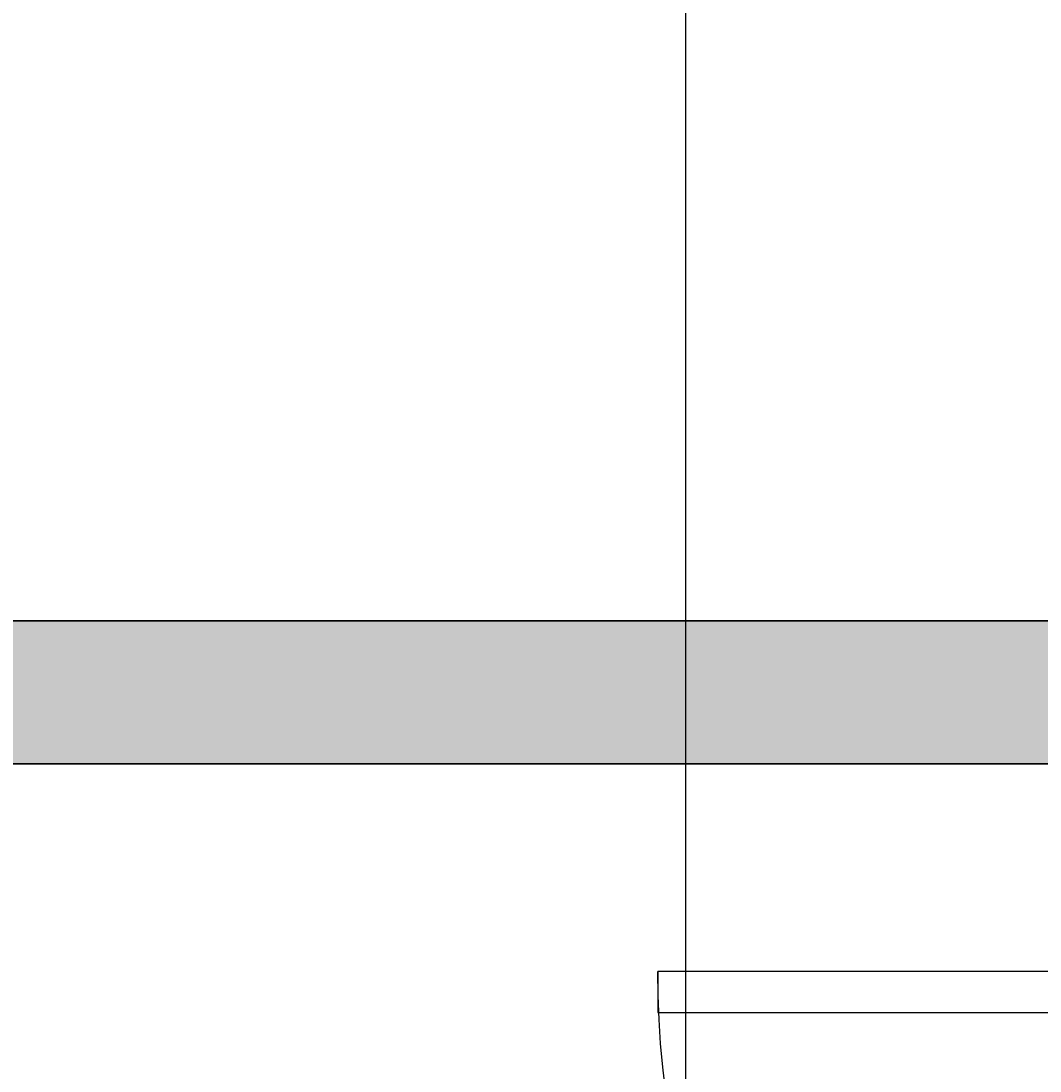
# Model space of a CAD drawing. Units: inches. Extents: x 1998 to 2588, y 1139 to 1977.
# Tile 65 of 134: x 2127 to 2160, y 1746 to 1779. Entities that reach past the tile are written whole.
import ezdxf

# ---------------------------------------------------------------- set-up
doc = ezdxf.new("R2010")
doc.units = ezdxf.units.IN
for name, color, linetype, lineweight in [('A-ANNO-DIMS', 2, 'Continuous', 18), ('A-WALL-PATT', 252, 'Continuous', 13), ('DOOR', 52, 'Continuous', 25), ('WALL', 200, 'Continuous', 35)]:
    doc.layers.add(name, color=color, linetype=linetype, lineweight=lineweight)
doc.styles.get("Standard").update_dxf_attribs({"font": 'arial.ttf'})
doc.dimstyles.get("Standard").update_dxf_attribs({"dimtxt": 0.18, "dimasz": 0.18, "dimexe": 0.18, "dimexo": 0.0625, "dimgap": 0.09, "dimtad": 0, "dimtih": 1, "dimtoh": 1, "dimdec": 4, "dimzin": 0, "dimdsep": 46, "dimtxsty": 'Standard', "dimcen": 0.09, "dimadec": 0, "dimazin": 0, "dimtfac": 1, "dimtdec": 4, "dimtofl": 0, "dimtmove": 0, "dimatfit": 3, "dimfxl": 1, "dimtolj": 1, "dimtzin": 0, "dimarcsym": 0})

# ---------------------------------------------------------------- blocks, each defined once
blk = doc.blocks.new('*U2')
for p, q in [((0, 0), (0, -6)), ((40, 0), (40, -6))]:
    blk.add_line(p, q)
blk.add_lwpolyline([(0, 0), (0, 40), (1.75, 40), (1.75, 0)], close=True)
blk.add_arc((0, 0), 40, 0, 90)
blk = doc.blocks.new('*D37')
at = {"layer": 'A-ANNO-DIMS', "color": 0, "lineweight": -2, "transparency": 16777216}
for p, q in [((2148.455, 1612.795), (2148.455, 1977.362)), ((2148.635, 1977.182), (2172.73, 1977.182)), ((2197.27, 1977.182), (2173.175, 1977.182)), ((2197.45, 1612.795), (2197.45, 1977.362))]:
    blk.add_line(p, q, dxfattribs=at)
at = {"layer": 'A-ANNO-DIMS', "color": 0, "transparency": 16777216}
for points in [[(2148.635, 1977.212), (2148.635, 1977.152), (2148.455, 1977.182)], [(2197.27, 1977.212), (2197.27, 1977.152), (2197.45, 1977.182)]]:
    blk.add_solid(points, dxfattribs=at)
at = {"layer": 'Defpoints', "color": 0, "transparency": 16777216}
for p in [(2197.45, 1977.182), (2148.455, 1612.732), (2197.45, 1612.732)]:
    blk.add_point(p, dxfattribs=at)
at = {"layer": 'A-ANNO-DIMS', "color": 0, "transparency": 16777216, "insert": (2172.952, 1977.182), "char_height": 0.18, "attachment_point": 5}
blk.add_mtext('\\A1;49', dxfattribs=at)

msp = doc.modelspace()

# ---------------------------------------------------------------- hatches: boundary and pattern name
at = {"layer": 'A-WALL-PATT'}
h = msp.add_hatch(color=256, dxfattribs=at)
h.dxf.hatch_style = 1
h.paths.add_polyline_path([(2222.9729, 1888.7324), (2099.4125, 1888.7324), (2099.4125, 1879.7324), (2222.9729, 1879.7324)])
h.paths.add_polyline_path([(2096.9729, 1868.3278), (2087.9729, 1868.3278), (2087.9729, 1775.637), (2096.9729, 1775.637)])
h.paths.add_polyline_path([(2227.4729, 1868.3278), (2222.9729, 1868.3278), (2222.9729, 1774.3318), (2227.4729, 1774.3318)])
h.paths.add_polyline_path([(2188.3019, 1759.7324), (2138.6074, 1759.7324), (2099.4125, 1759.7324), (2099.4125, 1755.2324), (2176.9729, 1755.2324), (2188.3019, 1755.2324)])
h.paths.add_polyline_path([(2087.9729, 1759.7324), (2059.4729, 1759.7324), (2059.4729, 1702.7324), (2087.9729, 1702.7324), (2087.9729, 1707.2324), (2063.9729, 1707.2324), (2063.9729, 1755.2324), (2087.9729, 1755.2324)])
h.paths.add_polyline_path([(2096.9729, 1755.2324), (2087.9729, 1755.2324), (2087.9729, 1707.2324), (2096.9729, 1707.2324)])
h.paths.add_polyline_path([(2187.0461, 1707.2324), (2105.9729, 1707.2324), (2096.9729, 1707.2324), (2087.9729, 1707.2324), (2087.9729, 1702.7324), (2105.9729, 1702.7324), (2114.9729, 1702.7324), (2187.0461, 1702.7324)])
h.paths.add_polyline_path([(2181.4729, 1719.2028), (2176.9729, 1719.2028), (2176.9729, 1707.2324), (2181.4729, 1707.2324)])
h.paths.add_polyline_path([(2216.0332, 1588.7324), (2114.9729, 1588.7324), (2105.9729, 1588.7324), (2105.9729, 1584.2324), (2216.0332, 1584.2324)])
h.paths.add_polyline_path([(2077.691, 1588.7324), (2061.4729, 1588.7324), (2061.4729, 1584.2324), (2077.691, 1584.2324)])
h.paths.add_polyline_path([(2105.9729, 1588.7324), (2098.0956, 1588.7324), (2098.0956, 1584.2324), (2105.9729, 1584.2324)])
h.paths.add_polyline_path([(2114.9729, 1596.2642), (2110.1012, 1596.2642), (2105.9729, 1596.2642), (2105.9729, 1588.7324), (2114.9729, 1588.7324)])
h.paths.add_polyline_path([(2114.9729, 1584.2324), (2105.9729, 1584.2324), (2105.9729, 1580.249), (2110.1012, 1580.249), (2114.9729, 1580.249)])
h.paths.add_polyline_path([(2114.9729, 1547.7716), (2110.1012, 1547.7716, -0.0318759), (2105.9729, 1548.035), (2105.9729, 1470.2324), (2108.3775, 1470.2324), (2108.3775, 1465.7324), (2186.2943, 1465.7324), (2186.2943, 1470.2324), (2114.9729, 1470.2324)])
h.paths.add_polyline_path([(2227.4729, 1584.2324), (2222.9729, 1584.2324), (2222.9729, 1486.137), (2227.4729, 1486.137)])
h.paths.add_polyline_path([(2295.4138, 1593.2324), (2227.4729, 1593.2324), (2227.4729, 1588.7324), (2295.4138, 1588.7324), (2295.4138, 1591.8729)])
h.paths.add_polyline_path([(2345.9729, 1627.1165), (2341.4729, 1627.1165), (2341.4729, 1593.2324), (2337.2869, 1593.2324), (2337.2869, 1591.8729), (2337.2869, 1588.7324), (2345.9729, 1588.7324)])
h.paths.add_polyline_path([(2291.9729, 1588.7324), (2287.4729, 1588.7324), (2287.4729, 1522.7324), (2291.9729, 1522.7324)])
h.paths.add_polyline_path([(2291.9729, 1522.7324), (2287.4729, 1522.7324), (2227.4729, 1522.7324), (2227.4729, 1518.2324), (2291.9729, 1518.2324)])
h.paths.add_polyline_path([(2295.7347, 1519.5919), (2295.7347, 1522.7324), (2291.9729, 1522.7324), (2291.9729, 1518.2324), (2295.7347, 1518.2324)])
h.paths.add_polyline_path([(2345.9729, 1522.7324), (2337.6078, 1522.7324), (2337.6078, 1519.5919), (2337.6078, 1518.2324), (2341.4729, 1518.2324), (2341.4729, 1488.5616), (2345.9729, 1488.5616)])
h.paths.add_polyline_path([(2345.9729, 1468.1569), (2341.4729, 1468.1569), (2341.4729, 1374.2324), (2227.4729, 1374.2324), (2227.4729, 1369.7324), (2345.9729, 1369.7324)])
h.paths.add_polyline_path([(2345.9729, 1369.7324), (2341.4729, 1369.7324), (2341.4729, 1362.2324), (2345.9729, 1362.2324)])
h.paths.add_polyline_path([(2345.9729, 1317.7324), (2345.9729, 1322.2324), (2341.4729, 1322.2324), (2341.4729, 1285.137), (2345.9729, 1285.137)], flags=17)
h.paths.add_polyline_path([(2356.2096, 1322.2324), (2345.9729, 1322.2324), (2345.9729, 1317.7324), (2356.2096, 1317.7324), (2356.2096, 1319.3088)], flags=17)
h.paths.add_polyline_path([(2393.9729, 1322.2324), (2375.6999, 1322.2324), (2375.6999, 1319.3088, -0.0202458), (2375.636, 1317.7324), (2393.9729, 1317.7324)], flags=17)
h.paths.add_polyline_path([(2398.4729, 1322.2324), (2393.9729, 1322.2324), (2393.9729, 1317.7324), (2393.9729, 1237.7324), (2345.9729, 1237.7324), (2345.9729, 1264.7324), (2341.4729, 1264.7324), (2341.4729, 1228.7324), (2393.9729, 1228.7324), (2482.7412, 1228.7324), (2482.7412, 1237.7324), (2398.4729, 1237.7324), (2398.4729, 1297.1029)])
h.paths.add_polyline_path([(2398.4729, 1362.2324), (2393.9729, 1362.2324), (2393.9729, 1357.7324), (2398.4729, 1357.7324)])
h.paths.add_polyline_path([(2345.9729, 1329.7549), (2341.4729, 1329.7549), (2341.4729, 1322.2324), (2345.9729, 1322.2324)])

# ---------------------------------------------------------------- linework, layer by layer
at = {"layer": 'WALL'}
for p, q in [((2099.4125, 1759.7324), (2138.6074, 1759.7324)), ((2138.6074, 1759.7324), (2188.3019, 1759.7324)), ((2087.9729, 1755.2324), (2138.6074, 1755.2324)), ((2096.9729, 1755.2324), (2176.9729, 1755.2324)), ((2138.6074, 1755.2324), (2188.3019, 1755.2324)), ((2188.3019, 1755.2324), (2138.6074, 1755.2324))]:
    msp.add_line(p, q, dxfattribs=at)

# ---------------------------------------------------------------- block references
at = {"layer": 'DOOR', "xscale": -0.736924595324625, "yscale": 0.736924595324625, "zscale": 0.736924595324625, "rotation": 90}
msp.add_blockref('*U2', (2177.0513, 1748.6798), dxfattribs=at)

# ---------------------------------------------------------------- dimensions: what is measured, and where the dimension line sits
at = {"layer": 'A-ANNO-DIMS'}
dim = msp.add_linear_dim(base=(2197.4499, 1977.1824), p1=(2148.4548, 1612.7324), p2=(2197.4499, 1612.7324), dimstyle='Standard', override={"dimdec": 0, "dimlfac": 1, "dimrnd": 0, "dimzin": 0, "dimdsep": 46, "dimlunit": 2}, dxfattribs=at)
dim.commit()
dim.dimension.update_dxf_attribs({"geometry": '*D37', "text_midpoint": (2172.9524, 1977.1824)})

doc.saveas('drawing.dxf')
